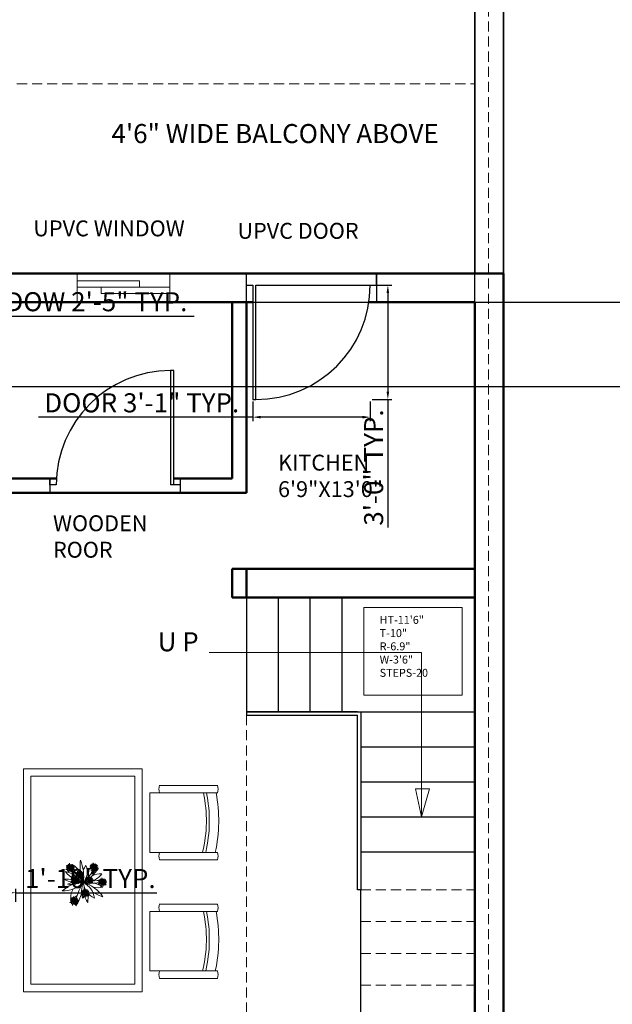
# Model space of a CAD drawing. Units: inches. Extents: x 2123 to 2977, y 1464 to 2698.
# Tile 8 of 10: x 2614 to 2801, y 2196 to 2506. Entities that reach past the tile are written whole.
import ezdxf

# ---------------------------------------------------------------- set-up
doc = ezdxf.new("R2010")
doc.units = ezdxf.units.IN
doc.linetypes.add('HIDDEN2', pattern=[4.7625, 3.175, -1.5875])
for name, color, linetype, lineweight in [('A-ANNO-DIMS', 2, 'Continuous', 18), ('A-ANNO-SYMB', 7, 'Continuous', 18), ('A-ANNO-TEXT', 7, 'Continuous', 18), ('A-AREA-IDEN', 7, 'Continuous', 25), ('A-DOOR', 4, 'Continuous', 25), ('A-FLOR-OVHD', 253, 'HIDDEN2', 18), ('A-FLOR-STRS', 7, 'Continuous', 25), ('A-FLOR-STRS-HIDN', 253, 'HIDDEN2', 18), ('A-FURN', 8, 'Continuous', 18), ('A-GLAZ', 4, 'Continuous', 18), ('A-WALL', 7, 'Continuous', 50), ('C-PROP', 21, 'HIDDEN2', 18), ('L-SITE-WALL', 7, 'Continuous', 35)]:
    doc.layers.add(name, color=color, linetype=linetype, lineweight=lineweight)
doc.styles.get("Standard").update_dxf_attribs({"font": 'arial.ttf'})
doc.dimstyles.new('ISO-25', dxfattribs={"dimtxt": 6, "dimasz": 2.5, "dimexe": 1.25, "dimexo": 0.625, "dimtad": 1, "dimdec": 0, "dimlunit": 3, "dimtxsty": 'Standard', "dimcen": 2.5, "dimadec": 0, "dimazin": 0, "dimtfac": 1, "dimtdec": 0, "dimtmove": 0, "dimatfit": 3, "dimfxl": 1, "dimarcsym": 0})

# ---------------------------------------------------------------- blocks, each defined once
blk = doc.blocks.new('*D9')
at = {"layer": 'A-ANNO-DIMS', "color": 0, "lineweight": -2, "transparency": 16777216}
for p, q in [((2767.56, 2548.37), (2808.58, 2548.37)), ((2807.33, 2545.87), (2807.33, 1686.46)), ((2767.56, 1683.96), (2808.58, 1683.96))]:
    blk.add_line(p, q, dxfattribs=at)
at = {"layer": 'A-ANNO-DIMS', "color": 0, "transparency": 16777216}
for points in [[(2806.91, 2545.87), (2807.74, 2545.87), (2807.33, 2548.37)], [(2806.91, 1686.46), (2807.74, 1686.46), (2807.33, 1683.96)]]:
    blk.add_solid(points, dxfattribs=at)
at = {"layer": 'Defpoints', "color": 0, "transparency": 16777216}
for p in [(2766.94, 2548.37), (2766.94, 1683.96), (2807.33, 1683.96)]:
    blk.add_point(p, dxfattribs=at)
at = {"layer": 'A-ANNO-DIMS', "color": 0, "transparency": 16777216, "insert": (2803.69, 2116.16), "char_height": 6, "attachment_point": 5, "rotation": 90}
blk.add_mtext("72'", dxfattribs=at)
blk = doc.blocks.new('DINING-CHAIR')
for p, q in [((0.42, 23.4), (18.64, 23.4)), ((0.39, 21.06), (21.73, 21.06)), ((21.73, 21.06), (21.73, 2.34)), ((18.66, 0), (0.38, 0)), ((21.73, 2.34), (0.43, 2.34))]:
    blk.add_line(p, q)
for centre, radius, start, end in [((3.85, 22.18), 3.64, 160.4535, 197.9116), ((15.19, 22.21), 3.64, 342.2774, 19.7376), ((46.03, 12.27), 46.04, 168.9982, 192.4562), ((46.66, 12.27), 43.7, 168.4012, 193.1346), ((46.66, 12.27), 42.76, 168.1438, 193.4274), ((3.85, 1.11), 3.64, 160.2624, 197.7226), ((15.19, 1.11), 3.64, 342.2774, 19.7376)]:
    blk.add_arc(centre, radius, start, end)
blk = doc.blocks.new('WINDOW-UPVC-29')
for p, q in [((0, 4.7), (0, 9)), ((0, 9), (0, 0)), ((19.61, 6.7), (0, 6.7)), ((19.61, 6.7), (19.61, 4.7)), ((29.17, 9), (29.17, 0)), ((29.17, 4.7), (0, 4.7)), ((7.53, 2.7), (7.53, 4.7)), ((29.17, 2.7), (7.53, 2.7))]:
    blk.add_line(p, q)
blk = doc.blocks.new('SWING-DOOR-36')
for p, q in [((37, 36), (36, 36)), ((36, 36), (36, 0)), ((37, 0), (37, 36))]:
    blk.add_line(p, q)
blk.add_arc((36, 0), 36, 90, 180)
blk = doc.blocks.new('*D35')
at = {"layer": 'A-ANNO-DIMS', "color": 0, "lineweight": -2, "transparency": 16777216}
for p, q in [((2591.21, 2228.06), (2591.21, 2232.2)), ((2613.29, 2228.06), (2613.29, 2232.2)), ((2593.71, 2230.95), (2610.79, 2230.95)), ((2613.29, 2230.95), (2657.71, 2230.95))]:
    blk.add_line(p, q, dxfattribs=at)
at = {"layer": 'A-ANNO-DIMS', "color": 0, "transparency": 16777216}
for points in [[(2593.71, 2231.37), (2593.71, 2230.53), (2591.21, 2230.95)], [(2610.79, 2231.37), (2610.79, 2230.53), (2613.29, 2230.95)]]:
    blk.add_solid(points, dxfattribs=at)
at = {"layer": 'Defpoints', "color": 0, "transparency": 16777216}
for p in [(2613.29, 2230.95), (2591.21, 2227.43), (2613.29, 2227.43)]:
    blk.add_point(p, dxfattribs=at)
at = {"layer": 'A-ANNO-DIMS', "color": 0, "transparency": 16777216, "insert": (2636.75, 2234.64), "char_height": 6, "attachment_point": 5}
blk.add_mtext('1\'-10" TYP.', dxfattribs=at)
blk = doc.blocks.new('*D38')
at = {"layer": 'A-ANNO-DIMS', "color": 0, "lineweight": -2, "transparency": 16777216}
for p, q in [((2687.94, 2385.58), (2687.94, 2379.41)), ((2724.94, 2385.58), (2724.94, 2379.41)), ((2687.94, 2380.66), (2620.44, 2380.66)), ((2722.44, 2380.66), (2690.44, 2380.66))]:
    blk.add_line(p, q, dxfattribs=at)
at = {"layer": 'A-ANNO-DIMS', "color": 0, "transparency": 16777216}
for points in [[(2690.44, 2381.08), (2690.44, 2380.24), (2687.94, 2380.66)], [(2722.44, 2381.08), (2722.44, 2380.24), (2724.94, 2380.66)]]:
    blk.add_solid(points, dxfattribs=at)
at = {"layer": 'Defpoints', "color": 0, "transparency": 16777216}
for p in [(2687.94, 2386.21), (2724.94, 2386.21), (2687.94, 2380.66)]:
    blk.add_point(p, dxfattribs=at)
at = {"layer": 'A-ANNO-DIMS', "color": 0, "transparency": 16777216, "insert": (2652.94, 2384.39), "char_height": 6, "attachment_point": 5}
blk.add_mtext('DOOR 3\'-1" TYP.', dxfattribs=at)
blk = doc.blocks.new('*D39')
at = {"layer": 'A-ANNO-DIMS', "color": 0, "lineweight": -2, "transparency": 16777216}
for p, q in [((2725.56, 2422.21), (2731.74, 2422.21)), ((2730.49, 2419.71), (2730.49, 2388.71)), ((2725.56, 2386.21), (2731.74, 2386.21)), ((2730.49, 2386.21), (2730.49, 2345.89))]:
    blk.add_line(p, q, dxfattribs=at)
at = {"layer": 'A-ANNO-DIMS', "color": 0, "transparency": 16777216}
for points in [[(2730.07, 2419.71), (2730.9, 2419.71), (2730.49, 2422.21)], [(2730.07, 2388.71), (2730.9, 2388.71), (2730.49, 2386.21)]]:
    blk.add_solid(points, dxfattribs=at)
at = {"layer": 'Defpoints', "color": 0, "transparency": 16777216}
for p in [(2724.94, 2422.21), (2724.94, 2386.21), (2730.49, 2386.21)]:
    blk.add_point(p, dxfattribs=at)
at = {"layer": 'A-ANNO-DIMS', "color": 0, "transparency": 16777216, "insert": (2726.79, 2364.8), "char_height": 6, "attachment_point": 5, "rotation": 90}
blk.add_mtext('3\'-0" TYP.', dxfattribs=at)
blk = doc.blocks.new('*D46')
at = {"layer": 'A-ANNO-DIMS', "color": 0, "lineweight": -2, "transparency": 16777216}
for p, q in [((2560.64, 2416.25), (2560.64, 2411.24)), ((2589.82, 2416.25), (2589.82, 2411.24)), ((2563.14, 2412.49), (2587.32, 2412.49)), ((2589.82, 2412.49), (2669.49, 2412.49))]:
    blk.add_line(p, q, dxfattribs=at)
at = {"layer": 'A-ANNO-DIMS', "color": 0, "transparency": 16777216}
for points in [[(2563.14, 2412.91), (2563.14, 2412.08), (2560.64, 2412.49)], [(2587.32, 2412.91), (2587.32, 2412.08), (2589.82, 2412.49)]]:
    blk.add_solid(points, dxfattribs=at)
at = {"layer": 'Defpoints', "color": 0, "transparency": 16777216}
for p in [(2560.64, 2416.87), (2589.82, 2416.87), (2589.82, 2412.49)]:
    blk.add_point(p, dxfattribs=at)
at = {"layer": 'A-ANNO-DIMS', "color": 0, "transparency": 16777216, "insert": (2630.9, 2416.22), "char_height": 6, "attachment_point": 5}
blk.add_mtext('WINDOW 2\'-5" TYP.', dxfattribs=at)
blk = doc.blocks.new('*D57')
at = {"layer": 'A-ANNO-DIMS', "color": 0, "lineweight": -2, "transparency": 16777216}
for p, q in [((2555.89, 1805.13), (2555.89, 2606.82)), ((2757.94, 1805.13), (2757.94, 2606.82)), ((2558.39, 2605.57), (2755.44, 2605.57))]:
    blk.add_line(p, q, dxfattribs=at)
at = {"layer": 'A-ANNO-DIMS', "color": 0, "transparency": 16777216}
for points in [[(2558.39, 2605.99), (2558.39, 2605.15), (2555.89, 2605.57)], [(2755.44, 2605.99), (2755.44, 2605.15), (2757.94, 2605.57)]]:
    blk.add_solid(points, dxfattribs=at)
at = {"layer": 'Defpoints', "color": 0, "transparency": 16777216}
for p in [(2757.94, 2605.57), (2555.89, 1804.5), (2757.94, 1804.5)]:
    blk.add_point(p, dxfattribs=at)
at = {"layer": 'A-ANNO-DIMS', "color": 0, "transparency": 16777216, "insert": (2656.91, 2609.26), "char_height": 6, "attachment_point": 5}
blk.add_mtext('16\'-10"', dxfattribs=at)
blk = doc.blocks.new('*D59')
at = {"layer": 'A-ANNO-DIMS', "color": 0, "lineweight": -2, "transparency": 16777216}
for p, q in [((2819.64, 2416.87), (2819.64, 2450.65)), ((2376.14, 2416.87), (2820.89, 2416.87)), ((2819.64, 2392.84), (2819.64, 2414.37)), ((2344.56, 2390.34), (2820.89, 2390.34))]:
    blk.add_line(p, q, dxfattribs=at)
at = {"layer": 'A-ANNO-DIMS', "color": 0, "transparency": 16777216}
for points in [[(2819.22, 2414.37), (2820.05, 2414.37), (2819.64, 2416.87)], [(2819.22, 2392.84), (2820.05, 2392.84), (2819.64, 2390.34)]]:
    blk.add_solid(points, dxfattribs=at)
at = {"layer": 'Defpoints', "color": 0, "transparency": 16777216}
for p in [(2375.52, 2416.87), (2819.64, 2416.87), (2343.94, 2390.34)]:
    blk.add_point(p, dxfattribs=at)
at = {"layer": 'A-ANNO-DIMS', "color": 0, "transparency": 16777216, "insert": (2815.91, 2435.01), "char_height": 6, "attachment_point": 5, "rotation": 90}
blk.add_mtext('2\'-2 1/2"', dxfattribs=at)

msp = doc.modelspace()

# ---------------------------------------------------------------- linework, layer by layer
at = {"layer": 'A-ANNO-SYMB'}
for p, q in [((2674.2, 2306.55), (2741.12, 2306.55)), ((2741.12, 2306.55), (2741.12, 2254.87)), ((2743.65, 2263.64), (2739.18, 2263.64)), ((2739.18, 2263.64), (2741.12, 2254.87)), ((2741.12, 2254.87), (2743.65, 2263.64))]:
    msp.add_line(p, q, dxfattribs=at)
at = {"layer": 'A-ANNO-TEXT'}
msp.add_lwpolyline([(2722.93, 2320.74), (2753.93, 2320.74), (2753.93, 2293.16), (2722.93, 2293.16)], close=True, dxfattribs=at)
at = {"layer": 'A-DOOR'}
for p, q in [((2685.94, 2416.87), (2685.94, 2425.87)), ((2726.94, 2422.21), (2726.94, 2425.87)), ((2726.94, 2425.87), (2726.94, 2416.87)), ((2685.94, 2422.21), (2687.94, 2422.21)), ((2688.94, 2422.21), (2724.94, 2422.21)), ((2724.94, 2422.21), (2726.94, 2422.21)), ((2624.01, 2359.33), (2624.01, 2361.37)), ((2624.01, 2361.37), (2624.01, 2356.87)), ((2626.01, 2359.33), (2624.01, 2359.33)), ((2663.01, 2359.33), (2662.01, 2359.33)), ((2665.01, 2359.33), (2663.01, 2359.33)), ((2665.01, 2361.37), (2665.01, 2356.87))]:
    msp.add_line(p, q, dxfattribs=at)
at = {"layer": 'A-FLOR-OVHD'}
msp.add_line((2589.82, 2485.57), (2757.94, 2485.57), dxfattribs=at)
at = {"layer": 'A-FLOR-STRS'}
for p, q in [((2685.94, 2323.87), (2685.94, 2287.87)), ((2695.94, 2323.87), (2695.94, 2287.87)), ((2705.94, 2323.87), (2705.94, 2287.87)), ((2715.94, 2323.87), (2715.94, 2287.87)), ((2685.94, 2287.87), (2721.94, 2287.87)), ((2720.94, 2287.87), (2685.94, 2287.87)), ((2685.94, 2287.87), (2685.94, 2286.87)), ((2721.94, 2287.87), (2757.94, 2287.87)), ((2721.94, 2287.87), (2721.94, 2231.87)), ((2685.94, 2286.87), (2720.94, 2286.87)), ((2720.94, 2231.87), (2720.94, 2286.87)), ((2721.94, 2276.87), (2757.94, 2276.87)), ((2721.94, 2265.87), (2757.94, 2265.87)), ((2721.94, 2254.87), (2757.94, 2254.87)), ((2721.94, 2243.87), (2757.94, 2243.87)), ((2721.94, 2231.87), (2720.94, 2231.87)), ((2721.94, 2191.87), (2721.94, 2231.87))]:
    msp.add_line(p, q, dxfattribs=at)
at = {"layer": 'A-FLOR-STRS-HIDN'}
for p, q in [((2685.94, 2286.87), (2685.94, 2191.87)), ((2721.94, 2231.87), (2757.94, 2231.87)), ((2721.94, 2221.87), (2757.94, 2221.87)), ((2721.94, 2211.87), (2757.94, 2211.87)), ((2721.94, 2201.87), (2757.94, 2201.87))]:
    msp.add_line(p, q, dxfattribs=at)
at = {"layer": 'A-FURN'}
for points in [[(2653.1, 2269.97), (2615.67, 2269.97), (2615.67, 2199.79), (2653.1, 2199.79)], [(2650.76, 2267.63), (2618.01, 2267.63), (2618.01, 2202.13), (2650.76, 2202.13)]]:
    msp.add_lwpolyline(points, close=True, dxfattribs=at)
for centre, radius, start, end in [((2647.43, 2239.32), 13.92, 172.3009, 189.7139), ((2620.73, 2235.97), 13.92, 352.3009, 22.0255), ((2630.32, 2236.9), 1.89, 89.1564, 133.4376), ((2629.05, 2240.17), 1.89, 269.1564, 313.4376), ((2630.16, 2241.3), 2.51, 245.3732, 274.4609), ((2629.3, 2236.51), 2.51, 65.3732, 94.4609), ((2630.72, 2240.65), 1.89, 217.8084, 258.7946), ((2628.85, 2237.63), 1.89, 60.6073, 78.7946), ((2630, 2237.08), 1.76, 78.4621, 111.5435), ((2629.71, 2240.43), 1.76, 258.4621, 268.2981), ((2631.73, 2240.97), 2.58, 211.2895, 237.5521), ((2628.15, 2237.46), 2.58, 31.2895, 57.5521), ((2630.49, 2237.87), 0.934, 145.6133, 182.6537), ((2629.42, 2238.75), 0.934, 278.5521, 306.3024), ((2628.84, 2238.68), 1.51, 4.4763, 53.7634), ((2631.24, 2240.01), 1.51, 184.4763, 205.3557), ((2632.46, 2237.3), 2.59, 144.6665, 178.9653), ((2627.76, 2238.84), 2.59, 324.6665, 343.9559), ((2632.93, 2239.84), 2.78, 172.3009, 189.7139), ((2627.59, 2239.17), 2.78, 352.3009, 22.0255), ((2631.76, 2238.24), 1.51, 158.5561, 197.2542), ((2628.91, 2238.35), 1.51, 338.5561, 17.2542), ((2631.25, 2239.21), 0.992, 138.0547, 156.7161), ((2629.61, 2239.46), 0.992, 318.0547, 24.4672), ((2628.5, 2241.74), 3.48, 302.0897, 323.7438), ((2633.15, 2236.74), 3.48, 122.0897, 143.7438), ((2631.31, 2235.49), 3.44, 82.5374, 106.1531), ((2630.8, 2242.21), 3.44, 262.5374, 286.1531), ((2631.54, 2238.92), 1.19, 185.896, 246.1019), ((2629.87, 2237.71), 1.19, 5.896, 66.1019), ((2629.76, 2236.66), 2.21, 34.2737, 74.5097), ((2632.05, 2238.52), 1.72, 195.5442, 214.4617), ((2623.51, 2227.41), 12.89, 31.2895, 57.5521), ((2641.44, 2244.98), 12.89, 211.2895, 237.5521), ((2631.84, 2238.67), 1.49, 124.9663, 145.8146), ((2628.93, 2237.82), 1.72, 350.7415, 11.1747), ((2629.5, 2240.02), 1.49, 331.3074, 355.3856), ((2631.48, 2237.92), 1.43, 88.5956, 113.6124), ((2632.18, 2240.04), 2.21, 236.3124, 254.5097), ((2630.39, 2240.23), 1.43, 293.4487, 322.2657), ((2631.27, 2239.99), 1.51, 258.7129, 281.758), ((2630.66, 2237.32), 1.51, 52.4708, 74.9809), ((2638.99, 2240.2), 7.56, 184.4763, 205.3557), ((2626.99, 2233.51), 7.56, 4.4763, 53.7634), ((2635.91, 2237.63), 2.78, 172.3009, 189.7139), ((2630.57, 2236.96), 2.78, 352.3009, 22.0255), ((2639.04, 2236.16), 4.96, 138.0547, 156.7161), ((2630.83, 2237.42), 4.96, 318.0547, 24.4672), ((2625.29, 2248.83), 17.38, 302.0897, 323.7438), ((2648.54, 2223.82), 17.38, 122.0897, 143.7438), ((2641.95, 2233.5), 7.45, 124.9663, 145.8146), ((2636.49, 2240.3), 1.89, 269.1564, 313.4376), ((2637.76, 2237.03), 1.89, 89.1564, 133.4376), ((2636.74, 2236.64), 2.51, 65.3732, 94.4609), ((2637.59, 2241.43), 2.51, 245.3732, 274.4609), ((2638.15, 2240.78), 1.89, 217.8084, 258.7946), ((2636.29, 2237.76), 1.89, 60.6073, 78.7946), ((2630.25, 2240.21), 7.45, 331.3074, 355.3856), ((2637.44, 2237.2), 1.76, 78.4621, 111.5435), ((2637.14, 2240.56), 1.76, 258.4621, 268.2981), ((2639.17, 2241.1), 2.58, 211.2895, 237.5521), ((2635.58, 2237.58), 2.58, 31.2895, 57.5521), ((2637.93, 2238), 0.934, 145.6133, 182.6537), ((2636.85, 2238.88), 0.934, 278.5521, 306.3024), ((2638.68, 2240.14), 1.51, 184.4763, 205.3557), ((2636.28, 2238.8), 1.51, 4.4763, 53.7634), ((2639.9, 2237.43), 2.59, 144.6665, 178.9653), ((2635.2, 2238.97), 2.59, 324.6665, 343.9559), ((2640.37, 2239.97), 2.78, 172.3009, 189.7139), ((2635.03, 2239.3), 2.78, 352.3009, 22.0255), ((2639.2, 2238.37), 1.51, 158.5561, 197.2542), ((2636.34, 2238.47), 1.51, 338.5561, 17.2542), ((2638.69, 2239.33), 0.992, 138.0547, 156.7161), ((2637.05, 2239.59), 0.992, 318.0547, 24.4672), ((2635.94, 2241.87), 3.48, 302.0897, 323.7438), ((2640.59, 2236.87), 3.48, 122.0897, 143.7438), ((2638.75, 2235.61), 3.44, 82.5374, 106.1531), ((2638.23, 2242.34), 3.44, 262.5374, 286.1531), ((2638.97, 2239.05), 1.19, 185.896, 246.1019), ((2637.3, 2237.83), 1.19, 5.896, 66.1019), ((2637.2, 2236.79), 2.21, 34.2737, 74.5097), ((2639.48, 2238.65), 1.72, 195.5442, 214.4617), ((2639.27, 2238.8), 1.49, 124.9663, 145.8146), ((2636.37, 2237.95), 1.72, 350.7415, 11.1747), ((2636.93, 2240.14), 1.49, 331.3074, 355.3856), ((2638.92, 2238.05), 1.43, 88.5956, 113.6124), ((2637.82, 2240.35), 1.43, 293.4487, 322.2657), ((2639.62, 2240.17), 2.21, 236.3124, 254.5097), ((2638.71, 2240.12), 1.51, 258.7129, 281.758), ((2638.09, 2237.44), 1.51, 52.4708, 74.9809), ((2629.29, 2222.69), 12.56, 65.3732, 94.4609), ((2633.55, 2246.62), 12.56, 245.3732, 274.4609), ((2636.36, 2243.39), 9.47, 217.8084, 258.7946), ((2627.04, 2228.3), 9.47, 60.6073, 78.7946), ((2630.54, 2236.15), 1.89, 269.1564, 313.4376), ((2631.81, 2232.88), 1.89, 89.1564, 133.4376), ((2630.79, 2232.49), 2.51, 65.3732, 94.4609), ((2631.64, 2237.27), 2.51, 245.3732, 274.4609), ((2632.21, 2236.63), 1.89, 217.8084, 258.7946), ((2630.34, 2233.61), 1.89, 60.6073, 78.7946), ((2631.49, 2233.05), 1.76, 78.4621, 111.5435), ((2633.22, 2236.95), 2.58, 211.2895, 237.5521), ((2629.63, 2233.43), 2.58, 31.2895, 57.5521), ((2630.33, 2234.65), 1.51, 4.4763, 53.7634), ((2632.73, 2235.99), 1.51, 184.4763, 205.3557), ((2633.95, 2233.27), 2.59, 144.6665, 178.9653), ((2634.42, 2235.82), 2.78, 172.3009, 189.7139), ((2629.08, 2235.14), 2.78, 352.3009, 22.0255), ((2633.25, 2234.22), 1.51, 158.5561, 197.2542), ((2630.39, 2234.32), 1.51, 338.5561, 17.2542), ((2632.74, 2235.18), 0.992, 138.0547, 156.7161), ((2631.1, 2235.43), 0.992, 318.0547, 24.4672), ((2629.99, 2237.72), 3.48, 302.0897, 323.7438), ((2634.64, 2232.72), 3.48, 122.0897, 143.7438), ((2632.8, 2231.46), 3.44, 82.5374, 106.1531), ((2632.29, 2238.19), 3.44, 262.5374, 286.1531), ((2633.02, 2234.89), 1.19, 185.896, 246.1019), ((2631.36, 2233.68), 1.19, 5.896, 66.1019), ((2631.25, 2232.64), 2.21, 34.2737, 74.5097), ((2632.02, 2237.96), 1.89, 269.1564, 313.4376), ((2633.3, 2234.69), 1.89, 89.1564, 133.4376), ((2632.28, 2234.3), 2.51, 65.3732, 94.4609), ((2633.13, 2239.09), 2.51, 245.3732, 274.4609), ((2633.32, 2234.65), 1.49, 124.9663, 145.8146), ((2631.83, 2235.43), 1.89, 60.6073, 78.7946), ((2633.69, 2238.44), 1.89, 217.8084, 258.7946), ((2630.98, 2235.99), 1.49, 331.3074, 355.3856), ((2632.97, 2234.87), 1.76, 78.4621, 111.5435), ((2632.68, 2238.22), 1.76, 258.4621, 268.2981), ((2632.97, 2233.89), 1.43, 88.5956, 113.6124), ((2631.87, 2236.2), 1.43, 293.4487, 322.2657), ((2634.71, 2238.76), 2.58, 211.2895, 237.5521), ((2631.12, 2235.25), 2.58, 31.2895, 57.5521), ((2633.46, 2235.66), 0.934, 145.6133, 182.6537), ((2632.39, 2236.54), 0.934, 278.5521, 306.3024), ((2632.15, 2233.29), 1.51, 52.4708, 74.9809), ((2634.22, 2237.81), 1.51, 184.4763, 205.3557), ((2631.82, 2236.47), 1.51, 4.4763, 53.7634), ((2635.44, 2235.09), 2.59, 144.6665, 178.9653), ((2630.74, 2236.63), 2.59, 324.6665, 343.9559), ((2634.73, 2236.03), 1.51, 158.5561, 197.2542), ((2631.88, 2236.14), 1.51, 338.5561, 17.2542), ((2634.23, 2237), 0.992, 138.0547, 156.7161), ((2632.59, 2237.25), 0.992, 318.0547, 24.4672), ((2631.48, 2239.53), 3.48, 302.0897, 323.7438), ((2636.13, 2234.53), 3.48, 122.0897, 143.7438), ((2634.28, 2233.28), 3.44, 82.5374, 106.1531), ((2633.77, 2240), 3.44, 262.5374, 286.1531), ((2634.51, 2236.71), 1.19, 185.896, 246.1019), ((2632.84, 2235.5), 1.19, 5.896, 66.1019), ((2632.73, 2234.45), 2.21, 34.2737, 74.5097), ((2635.02, 2236.31), 1.72, 195.5442, 214.4617), ((2634.81, 2236.47), 1.49, 124.9663, 145.8146), ((2631.91, 2235.62), 1.72, 350.7415, 11.1747), ((2632.47, 2237.81), 1.49, 331.3074, 355.3856), ((2634.46, 2235.71), 1.43, 88.5956, 113.6124), ((2633.36, 2238.02), 1.43, 293.4487, 322.2657), ((2635.15, 2237.83), 2.21, 236.3124, 254.5097), ((2634.25, 2237.79), 1.51, 258.7129, 281.758), ((2633.63, 2235.11), 1.51, 52.4708, 74.9809), ((2639.31, 2217.56), 17.22, 82.5374, 106.1531), ((2635, 2236.26), 1.89, 269.1564, 313.4376), ((2636.27, 2233), 1.89, 89.1564, 133.4376), ((2635.25, 2232.61), 2.51, 65.3732, 94.4609), ((2636.1, 2237.39), 2.51, 245.3732, 274.4609), ((2636.67, 2236.75), 1.89, 217.8084, 258.7946), ((2634.8, 2233.73), 1.89, 60.6073, 78.7946), ((2635.95, 2233.17), 1.76, 78.4621, 111.5435), ((2635.66, 2236.52), 1.76, 258.4621, 268.2981), ((2637.68, 2237.07), 2.58, 211.2895, 237.5521), ((2634.1, 2233.55), 2.58, 31.2895, 57.5521), ((2634.79, 2234.77), 1.51, 4.4763, 53.7634), ((2637.19, 2236.11), 1.51, 184.4763, 205.3557), ((2638.41, 2233.39), 2.59, 144.6665, 178.9653), ((2638.88, 2235.93), 2.78, 172.3009, 189.7139), ((2633.54, 2235.26), 2.78, 352.3009, 22.0255), ((2637.71, 2234.34), 1.51, 158.5561, 197.2542), ((2634.85, 2234.44), 1.51, 338.5561, 17.2542), ((2637.2, 2235.3), 0.992, 138.0547, 156.7161), ((2635.56, 2235.55), 0.992, 318.0547, 24.4672), ((2639.1, 2232.83), 3.48, 122.0897, 143.7438), ((2634.45, 2237.83), 3.48, 302.0897, 323.7438), ((2637.26, 2231.58), 3.44, 82.5374, 106.1531), ((2636.75, 2238.3), 3.44, 262.5374, 286.1531), ((2635.71, 2232.76), 2.21, 34.2737, 74.5097), ((2637.48, 2235.01), 1.19, 185.896, 246.1019), ((2635.82, 2233.8), 1.19, 5.896, 66.1019), ((2637.79, 2234.77), 1.49, 124.9663, 145.8146), ((2635.45, 2236.11), 1.49, 331.3074, 355.3856), ((2637.43, 2234.01), 1.43, 88.5956, 113.6124), ((2636.33, 2236.32), 1.43, 293.4487, 322.2657), ((2636.61, 2233.41), 1.51, 52.4708, 74.9809), ((2640.18, 2229.72), 7.16, 88.5956, 113.6124), ((2634.7, 2241.26), 7.16, 293.4487, 322.2657), ((2640.88, 2236.13), 1.89, 217.8084, 258.7946), ((2639.02, 2233.12), 1.89, 60.6073, 78.7946), ((2638.31, 2232.94), 2.58, 31.2895, 57.5521), ((2641.9, 2236.45), 2.58, 211.2895, 237.5521), ((2639.01, 2234.16), 1.51, 4.4763, 53.7634), ((2641.41, 2235.49), 1.51, 184.4763, 205.3557), ((2643.09, 2235.32), 2.78, 172.3009, 189.7139), ((2637.75, 2234.65), 2.78, 352.3009, 22.0255), ((2641.42, 2234.69), 0.992, 138.0547, 156.7161), ((2639.78, 2234.94), 0.992, 318.0547, 24.4672), ((2643.32, 2232.22), 3.48, 122.0897, 143.7438), ((2638.67, 2237.22), 3.48, 302.0897, 323.7438), ((2642, 2234.16), 1.49, 124.9663, 145.8146), ((2639.66, 2235.5), 1.49, 331.3074, 355.3856), ((2641.65, 2233.4), 1.43, 88.5956, 113.6124), ((2640.55, 2235.71), 1.43, 293.4487, 322.2657), ((2628.01, 2240.98), 9.47, 269.1564, 313.4376), ((2634.38, 2224.64), 9.47, 89.1564, 133.4376), ((2632.77, 2225.5), 8.78, 78.4621, 111.5435), ((2631.3, 2242.27), 8.78, 258.4621, 268.2981), ((2635.22, 2229.49), 4.67, 145.6133, 182.6537), ((2631.19, 2236.4), 1.76, 258.4621, 268.2981), ((2631.98, 2233.85), 0.934, 145.6133, 182.6537), ((2630.91, 2234.73), 0.934, 278.5521, 306.3024), ((2629.25, 2234.82), 2.59, 324.6665, 343.9559), ((2633.53, 2234.49), 1.72, 195.5442, 214.4617), ((2630.42, 2233.8), 1.72, 350.7415, 11.1747), ((2645.08, 2226.62), 12.94, 144.6665, 178.9653), ((2633.67, 2236.02), 2.21, 236.3124, 254.5097), ((2632.76, 2235.97), 1.51, 258.7129, 281.758), ((2641.56, 2231.34), 7.56, 158.5561, 197.2542), ((2636.44, 2232.99), 2.58, 211.2895, 237.5521), ((2632.86, 2229.48), 2.58, 31.2895, 57.5521), ((2627.3, 2231.86), 7.56, 338.5561, 17.2542), ((2633.55, 2230.7), 1.51, 4.4763, 53.7634), ((2635.95, 2232.03), 1.51, 184.4763, 205.3557), ((2636.76, 2251.18), 17.22, 262.5374, 286.1531), ((2640.45, 2234.71), 5.95, 185.896, 246.1019), ((2632.11, 2228.66), 5.95, 5.896, 66.1019), ((2631.57, 2223.44), 11.07, 34.2737, 74.5097), ((2637.64, 2231.86), 2.78, 172.3009, 189.7139), ((2632.3, 2231.19), 2.78, 352.3009, 22.0255), ((2635.96, 2231.23), 0.992, 138.0547, 156.7161), ((2634.32, 2231.48), 0.992, 318.0547, 24.4672), ((2633.21, 2233.76), 3.48, 302.0897, 323.7438), ((2637.86, 2228.76), 3.48, 122.0897, 143.7438), ((2636.55, 2230.7), 1.49, 124.9663, 145.8146), ((2636.44, 2233.97), 0.934, 145.6133, 182.6537), ((2635.37, 2234.85), 0.934, 278.5521, 306.3024), ((2634.21, 2232.04), 1.49, 331.3074, 355.3856), ((2633.71, 2234.94), 2.59, 324.6665, 343.9559), ((2637.99, 2234.61), 1.72, 195.5442, 214.4617), ((2634.88, 2233.92), 1.72, 350.7415, 11.1747), ((2638.13, 2236.14), 2.21, 236.3124, 254.5097), ((2637.22, 2236.09), 1.51, 258.7129, 281.758), ((2639.13, 2240.1), 7.56, 258.7129, 281.758), ((2636.06, 2226.7), 7.56, 52.4708, 74.9809), ((2639.21, 2235.65), 1.89, 269.1564, 313.4376), ((2640.49, 2232.38), 1.89, 89.1564, 133.4376), ((2640.32, 2236.78), 2.51, 245.3732, 274.4609), ((2639.47, 2231.99), 2.51, 65.3732, 94.4609), ((2640.16, 2232.56), 1.76, 78.4621, 111.5435), ((2639.87, 2235.91), 1.76, 258.4621, 268.2981), ((2640.65, 2233.35), 0.934, 145.6133, 182.6537), ((2639.58, 2234.23), 0.934, 278.5521, 306.3024), ((2642.62, 2232.78), 2.59, 144.6665, 178.9653), ((2637.93, 2234.32), 2.59, 324.6665, 343.9559), ((2641.92, 2233.72), 1.51, 158.5561, 197.2542), ((2639.07, 2233.83), 1.51, 338.5561, 17.2542), ((2641.47, 2230.97), 3.44, 82.5374, 106.1531), ((2640.96, 2237.69), 3.44, 262.5374, 286.1531), ((2641.7, 2234.4), 1.19, 185.896, 246.1019), ((2640.03, 2233.19), 1.19, 5.896, 66.1019), ((2639.92, 2232.14), 2.21, 34.2737, 74.5097), ((2642.21, 2234), 1.72, 195.5442, 214.4617), ((2639.1, 2233.3), 1.72, 350.7415, 11.1747), ((2642.34, 2235.52), 2.21, 236.3124, 254.5097), ((2641.43, 2235.47), 1.51, 258.7129, 281.758), ((2640.82, 2232.8), 1.51, 52.4708, 74.9809), ((2630.54, 2226.11), 2.51, 65.3732, 94.4609), ((2631.39, 2230.9), 2.51, 245.3732, 274.4609), ((2631.96, 2230.25), 1.89, 217.8084, 258.7946), ((2630.09, 2227.23), 1.89, 60.6073, 78.7946), ((2629.86, 2233.89), 4.67, 278.5521, 306.3024), ((2632.97, 2230.57), 2.58, 211.2895, 237.5521), ((2629.39, 2227.05), 2.58, 31.2895, 57.5521), ((2630.08, 2228.28), 1.51, 4.4763, 53.7634), ((2632.48, 2229.61), 1.51, 184.4763, 205.3557), ((2634.17, 2229.44), 2.78, 172.3009, 189.7139), ((2628.83, 2228.77), 2.78, 352.3009, 22.0255), ((2632.49, 2228.8), 0.992, 138.0547, 156.7161), ((2630.85, 2229.06), 0.992, 318.0547, 24.4672), ((2629.74, 2231.34), 3.48, 302.0897, 323.7438), ((2634.39, 2226.34), 3.48, 122.0897, 143.7438), ((2632.55, 2225.09), 3.44, 82.5374, 106.1531), ((2633.08, 2228.27), 1.49, 124.9663, 145.8146), ((2630.74, 2229.62), 1.49, 331.3074, 355.3856), ((2621.59, 2234.34), 12.94, 324.6665, 343.9559), ((2632.72, 2227.52), 1.43, 88.5956, 113.6124), ((2631.63, 2229.83), 1.43, 293.4487, 322.2657), ((2635.03, 2228.92), 1.89, 89.1564, 133.4376), ((2633.76, 2232.19), 1.89, 269.1564, 313.4376), ((2634.86, 2233.32), 2.51, 245.3732, 274.4609), ((2634.01, 2228.53), 2.51, 65.3732, 94.4609), ((2633.56, 2229.65), 1.89, 60.6073, 78.7946), ((2635.43, 2232.67), 1.89, 217.8084, 258.7946), ((2634.71, 2229.1), 1.76, 78.4621, 111.5435), ((2634.42, 2232.45), 1.76, 258.4621, 268.2981), ((2635.2, 2229.89), 0.934, 145.6133, 182.6537), ((2634.13, 2230.77), 0.934, 278.5521, 306.3024), ((2637.17, 2229.32), 2.59, 144.6665, 178.9653), ((2632.47, 2230.86), 2.59, 324.6665, 343.9559), ((2643, 2232.72), 8.59, 195.5442, 214.4617), ((2636.47, 2230.26), 1.51, 158.5561, 197.2542), ((2633.62, 2230.37), 1.51, 338.5561, 17.2542), ((2636.02, 2227.51), 3.44, 82.5374, 106.1531), ((2635.51, 2234.23), 3.44, 262.5374, 286.1531), ((2636.24, 2230.94), 1.19, 185.896, 246.1019), ((2634.58, 2229.73), 1.19, 5.896, 66.1019), ((2634.47, 2228.68), 2.21, 34.2737, 74.5097), ((2636.76, 2230.54), 1.72, 195.5442, 214.4617), ((2633.64, 2229.84), 1.72, 350.7415, 11.1747), ((2636.19, 2229.94), 1.43, 88.5956, 113.6124), ((2635.1, 2232.25), 1.43, 293.4487, 322.2657), ((2636.89, 2232.06), 2.21, 236.3124, 254.5097), ((2635.98, 2232.01), 1.51, 258.7129, 281.758), ((2635.37, 2229.34), 1.51, 52.4708, 74.9809), ((2627.44, 2229.24), 8.59, 350.7415, 11.1747), ((2643.67, 2240.34), 11.07, 236.3124, 254.5097), ((2630.29, 2229.77), 1.89, 269.1564, 313.4376), ((2631.56, 2226.5), 1.89, 89.1564, 133.4376), ((2631.24, 2226.67), 1.76, 78.4621, 111.5435), ((2630.95, 2230.03), 1.76, 258.4621, 268.2981), ((2631.73, 2227.47), 0.934, 145.6133, 182.6537), ((2630.66, 2228.35), 0.934, 278.5521, 306.3024), ((2633.7, 2226.9), 2.59, 144.6665, 178.9653), ((2629, 2228.44), 2.59, 324.6665, 343.9559), ((2633, 2227.84), 1.51, 158.5561, 197.2542), ((2630.15, 2227.95), 1.51, 338.5561, 17.2542), ((2632.04, 2231.81), 3.44, 262.5374, 286.1531), ((2631, 2226.26), 2.21, 34.2737, 74.5097), ((2632.77, 2228.52), 1.19, 185.896, 246.1019), ((2631.11, 2227.31), 1.19, 5.896, 66.1019), ((2633.29, 2228.12), 1.72, 195.5442, 214.4617), ((2630.17, 2227.42), 1.72, 350.7415, 11.1747), ((2633.42, 2229.64), 2.21, 236.3124, 254.5097), ((2632.51, 2229.59), 1.51, 258.7129, 281.758), ((2631.9, 2226.91), 1.51, 52.4708, 74.9809)]:
    msp.add_arc(centre, radius, start, end, dxfattribs=at)
at = {"layer": 'A-GLAZ'}
msp.add_line((2661.82, 2416.87), (2661.82, 2416.87), dxfattribs=at)
at = {"layer": 'A-WALL'}
for p, q in [((2250.94, 2425.87), (2766.94, 2425.87)), ((2766.94, 2425.87), (2766.94, 1897.87)), ((2250.94, 2416.87), (2687.94, 2416.87)), ((2681.44, 2416.87), (2681.44, 2361.37)), ((2685.94, 2416.87), (2685.94, 2356.87)), ((2724.54, 2416.87), (2757.94, 2416.87)), ((2757.94, 2416.87), (2757.94, 1897.87)), ((2537.44, 2361.37), (2626.06, 2361.37)), ((2663.01, 2361.37), (2681.44, 2361.37)), ((2681.44, 2361.37), (2681.44, 2361.37)), ((2681.44, 2361.37), (2681.44, 2361.37)), ((2537.44, 2356.87), (2685.94, 2356.87)), ((2681.44, 2332.87), (2681.44, 2323.87)), ((2681.44, 2332.87), (2757.94, 2332.87)), ((2685.94, 2332.87), (2685.94, 2323.87)), ((2681.44, 2323.87), (2757.94, 2323.87))]:
    msp.add_line(p, q, dxfattribs=at)
at = {"layer": 'C-PROP'}
msp.add_line((2762.16, 2552.87), (2762.16, 1683.96), dxfattribs=at)
at = {"layer": 'L-SITE-WALL'}
for p, q in [((2766.94, 2425.87), (2766.94, 2552.87)), ((2757.94, 2425.87), (2757.94, 2543.87))]:
    msp.add_line(p, q, dxfattribs=at)

# ---------------------------------------------------------------- block references
at = {"layer": 'A-DOOR', "rotation": 180}
msp.add_blockref('SWING-DOOR-36', (2724.94, 2422.21), dxfattribs=at)
at = {"layer": 'A-DOOR'}
msp.add_blockref('SWING-DOOR-36', (2626.01, 2359.33), dxfattribs=at)
at = {"layer": 'A-FURN', "extrusion": (0, 0, -1), "zscale": -1}
for p in [(-2677.2, 2241.33), (-2677.2, 2203.99)]:
    msp.add_blockref('DINING-CHAIR', p, dxfattribs=at)
at = {"layer": 'A-GLAZ'}
msp.add_blockref('WINDOW-UPVC-29', (2632.64, 2416.87), dxfattribs=at)

# ---------------------------------------------------------------- texts
at = {"layer": 'A-ANNO-SYMB', "insert": (2657.96, 2312.96), "char_height": 6, "attachment_point": 1}
msp.add_mtext_dynamic_manual_height_columns('U P', width=158.0108, gutter_width=12.5, heights=[0], dxfattribs=at)
at = {"layer": 'A-ANNO-TEXT', "attachment_point": 1}
for s, width, insert, char_height in [('4\'6" WIDE BALCONY ABOVE', 209.2537, (2643.43, 2472.93), 6), ('UPVC WINDOW', 116.1895, (2618.78, 2442.58), 5), ('UPVC DOOR', 116.1895, (2683.09, 2441.81), 5), ('WOODEN \\PROOR', 69.1443, (2624.98, 2349.76), 5), ('HT-11\'6"\\PT-10"\\PR-6.9"\\PW-3\'6"\\PSTEPS-20', 87.3392, (2727.91, 2318.1), 2.5)]:
    msp.add_mtext_dynamic_manual_height_columns(s, width=width, gutter_width=12.5, heights=[0], dxfattribs=dict(at, insert=insert, char_height=char_height))
at = {"layer": 'A-AREA-IDEN', "insert": (2695.88, 2368.84), "char_height": 5, "attachment_point": 1}
msp.add_mtext_dynamic_manual_height_columns('KITCHEN\\P6\'9"X13\'0"', width=106.3581, gutter_width=12.5, heights=[0], dxfattribs=at)

# ---------------------------------------------------------------- dimensions: what is measured, and where the dimension line sits
at = {"layer": 'A-ANNO-DIMS'}
dim = msp.add_linear_dim(base=(2757.9353, 2605.5708), p1=(2555.8869, 1804.5032), p2=(2757.9353, 1804.5032), dimstyle='ISO-25', override={"dimdec": 1, "dimlfac": 1, "dimrnd": 0, "dimzin": 1, "dimdsep": 46, "dimlunit": 4, "dimfrac": 2}, dxfattribs=at)
dim.commit()
dim.dimension.update_dxf_attribs({"geometry": '*D57', "text_midpoint": (2656.9111, 2609.2592)})
for base, p1, p2, override, picture, middle in [((2807.33, 1683.96), (2766.94, 2548.37), (2766.94, 1683.96), {"dimclrd": 0, "dimclre": 0, "dimclrt": 0}, '*D9', (2803.69, 2116.16)), ((2819.64, 2416.87), (2343.94, 2390.34), (2375.52, 2416.87), {"dimdec": 1, "dimlfac": 1, "dimrnd": 0, "dimzin": 1, "dimdsep": 46, "dimlunit": 4, "dimfrac": 2}, '*D59', (2815.91, 2435.01))]:
    dim = msp.add_linear_dim(base=base, p1=p1, p2=p2, angle=90, dimstyle='ISO-25', override=override, dxfattribs=at)
    dim.commit()
    dim.dimension.update_dxf_attribs({"geometry": picture, "text_midpoint": middle})
for base, p1, p2, text, picture, middle in [((2589.82, 2412.49), (2560.64, 2416.87), (2589.82, 2416.87), 'WINDOW <> TYP.', '*D46', (2630.9, 2416.22)), ((2613.29, 2230.95), (2591.21, 2227.43), (2613.29, 2227.43), '<> TYP.', '*D35', (2636.75, 2234.64))]:
    dim = msp.add_linear_dim(base=base, p1=p1, p2=p2, text=text, dimstyle='ISO-25', override={"dimdec": 1, "dimlfac": 1, "dimrnd": 0, "dimzin": 1, "dimdsep": 46, "dimlunit": 4, "dimfrac": 2}, dxfattribs=at)
    dim.commit()
    dim.dimension.update_dxf_attribs({"geometry": picture, "text_midpoint": middle})
for base, p1, p2, angle, text, picture, middle in [((2730.49, 2386.21), (2724.94, 2422.21), (2724.94, 2386.21), 270, '<> TYP.', '*D39', (2726.79, 2364.8)), ((2687.94, 2380.66), (2724.94, 2386.21), (2687.94, 2386.21), 180, 'DOOR <> TYP.', '*D38', (2652.94, 2384.39))]:
    dim = msp.add_linear_dim(base=base, p1=p1, p2=p2, angle=angle, text=text, dimstyle='ISO-25', override={"dimdec": 1, "dimlfac": 1, "dimrnd": 0, "dimzin": 1, "dimdsep": 46, "dimlunit": 4, "dimfrac": 2}, dxfattribs=at)
    dim.commit()
    dim.dimension.update_dxf_attribs({"geometry": picture, "text_midpoint": middle})

doc.saveas('drawing.dxf')
